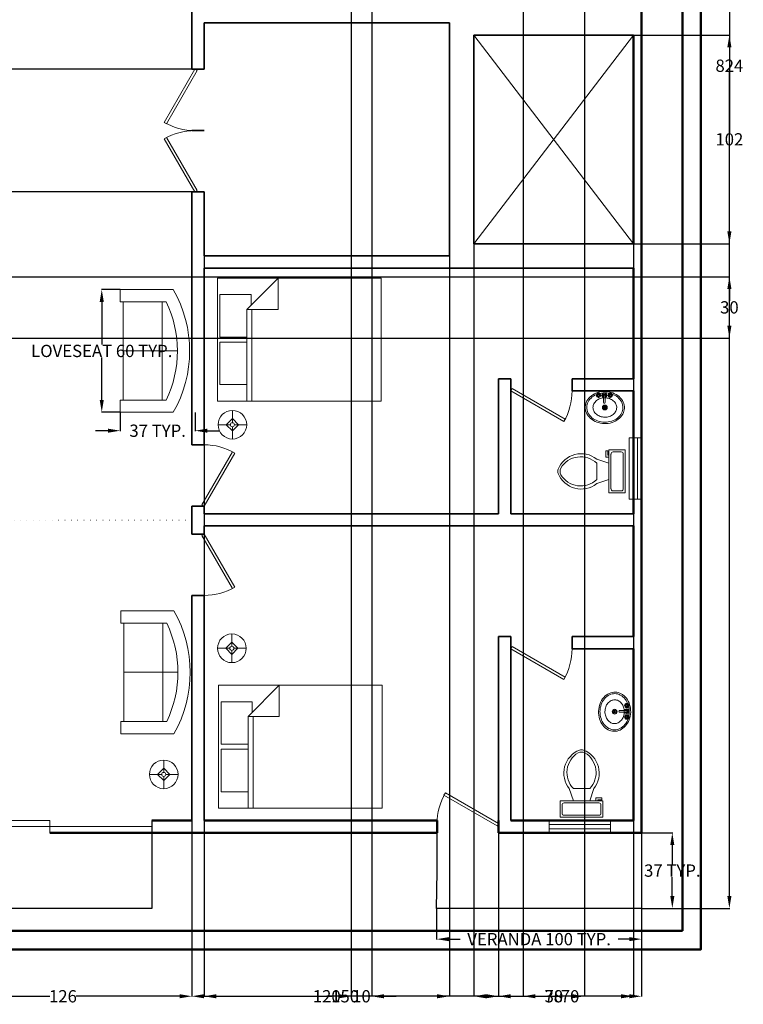
# Model space of a CAD drawing. Units: inches. Extents: x 910 to 1553, y 598 to 1516.
# Tile 2 of 6: x 1198 to 1551, y 598 to 1079. Entities that reach past the tile are written whole.
import ezdxf

# ---------------------------------------------------------------- set-up
doc = ezdxf.new("R2010")
doc.units = ezdxf.units.IN
doc.header["$MEASUREMENT"] = 0
doc.linetypes.add('ACAD_ISO07W100', pattern=[3, 0, -3])
for name, color, linetype, lineweight in [('A-ANNO-DIMS', 2, 'Continuous', 18), ('A-FLOR-BALC', 8, 'Continuous', 25), ('A-FLOR-OPEN', 8, 'Continuous', 13), ('A-FLOR-OVHD', 8, 'ACAD_ISO07W100', 13), ('doors', 2, 'Continuous', 18), ('furniture', 11, 'Continuous', 18), ('Inner wall', 230, 'Continuous', 35), ('outer wall', 231, 'Continuous', 50), ('sanitory', 141, 'Continuous', 18), ('windows', 6, 'Continuous', 18)]:
    doc.layers.add(name, color=color, linetype=linetype, lineweight=lineweight)
doc.styles.get("Standard").update_dxf_attribs({"font": 'arial.ttf'})
doc.dimstyles.get("Standard").update_dxf_attribs({"dimtxt": 6, "dimasz": 6, "dimexe": 0.18, "dimexo": 0.0625, "dimgap": 0.09, "dimtad": 0, "dimtih": 1, "dimtoh": 1, "dimdec": 0, "dimzin": 0, "dimdsep": 46, "dimlunit": 3, "dimtxsty": 'Standard', "dimcen": 0.09, "dimadec": 0, "dimazin": 0, "dimtfac": 1, "dimtdec": 0, "dimtofl": 0, "dimtmove": 0, "dimatfit": 3, "dimfxl": 1, "dimtolj": 1, "dimtzin": 0, "dimarcsym": 0})

# ---------------------------------------------------------------- blocks, each defined once
blk = doc.blocks.new('*U5')
for p, q in [((0, 0), (0, -6)), ((-40, 0), (-40, -6))]:
    blk.add_line(p, q)
blk.add_lwpolyline([(0, 0), (-34.64, 20), (-35.52, 18.48), (-0.88, -1.52)], close=True)
blk.add_arc((0, 0), 40, 150, 180)
blk = doc.blocks.new('*U4')
for p, q in [((0, 0), (0, 6)), ((40, 0), (40, 6))]:
    blk.add_line(p, q)
blk.add_lwpolyline([(0, 0), (34.64, -20), (35.52, -18.48), (0.87, 1.52)], close=True)
blk.add_arc((0, 0), 40, 330, 0)
blk = doc.blocks.new('*U8')
for p, q in [((0, 0), (0, 6)), ((40, 0), (40, 6))]:
    blk.add_line(p, q)
blk.add_lwpolyline([(0, 0), (34.64, -20), (35.52, -18.48), (0.88, 1.52)], close=True)
blk.add_arc((0, 0), 40, 330, 360)
blk = doc.blocks.new('*U6')
for p, q in [((-40, 0), (-40, 6)), ((0, 0), (0, 6))]:
    blk.add_line(p, q)
blk.add_lwpolyline([(0, 0), (-34.64, -20), (-35.52, -18.48), (-0.88, 1.52)], close=True)
blk.add_arc((0, 0), 40, 180, 210)
blk = doc.blocks.new('*U2')
for p, q in [((0, 0), (0, -6)), ((40, 0), (40, -6))]:
    blk.add_line(p, q)
blk.add_lwpolyline([(0, 0), (34.64, 20), (35.52, 18.48), (0.87, -1.52)], close=True)
blk.add_arc((0, 0), 40, 0, 30)
blk = doc.blocks.new('Bed - Queen')
for p, q in [((0, -80.00003), (0, 0)), ((0, 0), (59.99999, 0)), ((59.99999, 0), (59.99999, -80.00003)), ((7.99999, -1.2), (28.79998, -1.2)), ((7.99999, -14.4), (7.99999, -1.2)), ((28.79998, -1.2), (28.79998, -14.4)), ((31.19999, -1.2), (51.99999, -1.2)), ((31.19999, -14.4), (31.19999, -1.2)), ((51.99999, -1.2), (51.99999, -16.4)), ((0, -14.4), (44.8, -14.4)), ((59.99999, -29.6), (44.8, -14.4)), ((44.8, -14.4), (44.8, -29.6)), ((44.8, -16.8), (0, -16.8)), ((51.99999, -16.4), (46.79936, -16.4)), ((44.8, -29.6), (59.99999, -29.6)), ((59.99999, -80.00003), (0, -80.00003))]:
    blk.add_line(p, q)
blk = doc.blocks.new('Lamp - Table')
for p, q in [((0, 7), (0, 1)), ((-1, 0), (-7, 0)), ((0, 3), (-3, 0)), ((-3, 0), (0, -3)), ((3, 0), (0, 3)), ((0, -3), (3, 0)), ((1, 0), (7, 0)), ((0, -1), (0, -7))]:
    blk.add_line(p, q)
for radius in [7, 1]:
    blk.add_circle((0, 0), radius)
blk = doc.blocks.new('Toilet - top')
for p, q in [((9.5, -6), (9.5, -2)), ((-10, -8.5), (-8, -8.5)), ((-10, -9.5), (-10, -8.5)), ((-7, -9.5), (-10, -9.5)), ((-8, -8.5), (-8, -8)), ((-7, -8), (-7, -9.5)), ((-4, -8), (-6, -14)), ((4, -8), (6, -14)), ((4, -14), (-4, -14))]:
    blk.add_line(p, q)
blk.add_lwpolyline([(10.5, -8), (10.5, 0), (-10.5, 0), (-10.5, -8)], close=True)
for points in [[(-9.5, -2), (-9.5, -6)], [(8.5, -1), (-8.5, -1)], [(-8.5, -7), (8.5, -7)]]:
    blk.add_lwpolyline(points)
for centre, radius, start, end in [((-8.62, -1.88), 0.884, 81.8699, 188.1301), ((8.62, -1.88), 0.884, 351.8699, 98.1301), ((-8.62, -6.12), 0.884, 171.8699, 278.1301), ((8.62, -6.12), 0.884, 261.8699, 8.1301), ((3.52, -21.58), 12.17, 141.4691, 247.9714), ((4.2, -21.82), 11.33, 136.3677, 238.9468), ((-3.52, -21.58), 12.17, 292.0284, 38.5307), ((-4.2, -21.82), 11.33, 301.053, 43.6321), ((0, -27.88), 4, 245.7318, 294.2682), ((0, -29), 4, 254.8605, 285.1395)]:
    blk.add_arc(centre, radius, start, end)
blk = doc.blocks.new('Sofa - Roundback Loveseat 5 ft.')
for p, q in [((0, -32.44198), (0, -5.99998)), ((-24, -33.99998), (-24, -11.46958)), ((-23.9998, -13.38178), (23.99986, -13.38178)), ((24.00004, -33.99998), (24.00004, -11.46958)), ((-24, -32.44198), (24.00004, -32.44198))]:
    blk.add_line(p, q)
for points in [[(-24, -33.99998), (-30, -33.99998), (-30, -7.99998)], [(30.00004, -7.99998), (30.00004, -33.99998), (24.00004, -33.99998)]]:
    blk.add_lwpolyline(points)
for centre, radius, start, end in [((0, -60.24998), 60.24998, 60.13715, 119.8628), ((0, -61.38438), 55.38444, 64.32083, 115.6792)]:
    blk.add_arc(centre, radius, start, end)
blk = doc.blocks.new('Faucet - Bathroom top')
for p, q in [((-4.107, 0.125), (-4.375, 0.125)), ((-3.75, 0.4788), (-3.75, 0.75)), ((-3.5, 0.482), (-3.5, 0.75)), ((-3.1461, 0.125), (-2.875, 0.125)), ((3.143, 0.125), (2.875, 0.125)), ((3.5, 0.4788), (3.5, 0.75)), ((3.75, 0.482), (3.75, 0.75)), ((4.1039, 0.125), (4.375, 0.125)), ((-4.1039, -0.125), (-4.375, -0.125)), ((-3.75, -0.4821), (-3.75, -0.75)), ((-3.5, -0.4789), (-3.5, -0.75)), ((-3.143, -0.125), (-2.875, -0.125)), ((-0.5, -0.8639), (-0.5, -4.5)), ((0.5, -4.5), (0.5, -0.8631)), ((3.1461, -0.125), (2.875, -0.125)), ((3.5, -0.4821), (3.5, -0.75)), ((3.75, -0.4789), (3.75, -0.75)), ((4.107, -0.125), (4.375, -0.125))]:
    blk.add_line(p, q)
for centre, radius in [((-3.625, 0), 1.375), ((-4.625, 0), 0.2795), ((-3.625, 0), 0.5), ((-3.625, 1), 0.2795), ((-2.625, 0), 0.2795), ((0, 0), 0.5), ((3.625, 0), 1.375), ((2.625, 0), 0.2795), ((3.625, 0), 0.5), ((3.625, 1), 0.2795), ((4.625, 0), 0.2795), ((-3.625, -1), 0.2795), ((3.625, -1), 0.2795)]:
    blk.add_circle(centre, radius)
for centre, radius, start, end in [((-3.625, 0), 1, 105.2407, 164.2093), ((-3.625, 0), 1, 16.44125, 74.07887), ((0, 0), 1.5, 289.6514, 250.3603), ((0, 0), 1, 300.3431, 239.7554), ((3.625, 0), 1, 106.12, 164.0884), ((3.625, 0), 1, 16.23422, 73.90469), ((-3.625, 0), 1, 196.2342, 253.9047), ((-3.625, 0), 1, 286.12, 344.0884), ((0, -4.5), 0.5, 180, 0), ((3.625, 0), 1, 196.4413, 254.0789), ((3.625, 0), 1, 285.2407, 344.2093)]:
    blk.add_arc(centre, radius, start, end)
blk = doc.blocks.new('Sink - Oval top')
for p, q in [((-1, 0), (1, 0)), ((0, 1), (0, -1))]:
    blk.add_line(p, q)
for points in [[(-12.23, 0.39, 0.117634), (-11.46, -3.36, 0.104469), (-8.88, -6.8, 0.090016), (-5.08, -9.07, 0.08192), (-0.32, -10.02, 0.08192), (4.49, -9.38, 0.090016), (8.42, -7.36, 0.104469), (11.22, -4.09, 0.117634), (12.23, -0.39, 0.117634), (11.46, 3.36, 0.104469), (8.88, 6.8, 0.090016), (5.08, 9.07, 0.08192), (0.32, 10.02, 0.08192), (-4.49, 9.38, 0.090016), (-8.42, 7.36, 0.104469), (-11.22, 4.09, 0.117634)], [(-11.29, 0.16, 0.118622), (-10.52, -3.25, 0.104678), (-8.07, -6.36, 0.089562), (-4.54, -8.37, 0.081185), (-0.13, -9.15, 0.081185), (4.3, -8.49, 0.089562), (7.89, -6.58, 0.104678), (10.42, -3.55, 0.118622), (11.29, -0.16, 0.118622), (10.52, 3.25, 0.104678), (8.07, 6.36, 0.089562), (4.54, 8.37, 0.081185), (0.13, 9.15, 0.081185), (-4.3, 8.49, 0.089562), (-7.89, 6.58, 0.104678), (-10.42, 3.55, 0.118622)], [(-7.42, 0.08, 0.118283), (-6.91, -2.17, 0.104607), (-5.29, -4.21, 0.089718), (-2.97, -5.53, 0.081436), (-0.07, -6.04, 0.081436), (2.84, -5.59, 0.089718), (5.2, -4.33, 0.104607), (6.86, -2.32, 0.118283), (7.42, -0.08, 0.118283), (6.91, 2.17, 0.104607), (5.29, 4.21, 0.089718), (2.97, 5.53, 0.081436), (0.07, 6.04, 0.081436), (-2.84, 5.59, 0.089718), (-5.2, 4.33, 0.104607), (-6.86, 2.32, 0.118283)]]:
    blk.add_lwpolyline(points, format="xyb", close=True)
for radius in [1.5, 1]:
    blk.add_circle((0, 0), radius)
blk = doc.blocks.new('WIN-30X6')
for p, q in [((0, 6), (30, 6)), ((0, 0), (0, 6)), ((30, 6), (30, 0)), ((0, 4), (30, 4)), ((30, 2), (0, 2)), ((30, 0), (0, 0))]:
    blk.add_line(p, q)
blk = doc.blocks.new('VERANDA-EDGE-DEEP')
for p, q in [((0.23, 17.99), (0.23, 36.98)), ((100.23, 36.98), (100.23, 17.99)), ((0, 0), (0.23, 17.99)), ((100.23, 17.99), (100.23, 0)), ((100.23, 0), (0, 0))]:
    blk.add_line(p, q)
blk = doc.blocks.new('*D41')
at = {"layer": 'A-ANNO-DIMS', "color": 0, "lineweight": -2, "transparency": 16777216}
for p, q in [((1246.6, 947.53), (1237.49, 947.53)), ((1237.67, 941.53), (1237.67, 920.72)), ((1237.67, 893.53), (1237.67, 914.33)), ((1246.6, 887.53), (1237.49, 887.53))]:
    blk.add_line(p, q, dxfattribs=at)
for points in [[(1236.67, 941.53), (1238.67, 941.53), (1237.67, 947.53)], [(1236.67, 893.53), (1238.67, 893.53), (1237.67, 887.53)]]:
    blk.add_solid(points, dxfattribs=at)
at = {"layer": 'Defpoints', "color": 0, "lineweight": -2, "transparency": 16777216}
for p in [(1246.67, 947.53), (1237.67, 887.53), (1246.67, 887.53)]:
    blk.add_point(p, dxfattribs=at)
at = {"layer": 'A-ANNO-DIMS', "color": 0, "transparency": 16777216, "insert": (1237.67, 917.53), "char_height": 6, "attachment_point": 5}
blk.add_mtext('\\A1;LOVESEAT 60 TYP.', dxfattribs=at)
blk = doc.blocks.new('*D42')
at = {"layer": 'A-ANNO-DIMS', "color": 0, "lineweight": -2, "transparency": 16777216}
for p, q in [((1246.67, 887.46), (1246.67, 878.35)), ((1283.33, 887.46), (1283.33, 878.35)), ((1240.67, 878.53), (1234.67, 878.53)), ((1289.33, 878.53), (1295.33, 878.53))]:
    blk.add_line(p, q, dxfattribs=at)
for points in [[(1240.67, 879.53), (1240.67, 877.53), (1246.67, 878.53)], [(1289.33, 879.53), (1289.33, 877.53), (1283.33, 878.53)]]:
    blk.add_solid(points, dxfattribs=at)
at = {"layer": 'Defpoints', "color": 0, "lineweight": -2, "transparency": 16777216}
for p in [(1246.67, 887.53), (1283.33, 887.53), (1283.33, 878.53)]:
    blk.add_point(p, dxfattribs=at)
at = {"layer": 'A-ANNO-DIMS', "color": 0, "transparency": 16777216, "insert": (1265, 878.53), "char_height": 6, "attachment_point": 5}
blk.add_mtext('\\A1;37 TYP.', dxfattribs=at)
blk = doc.blocks.new('*D47')
at = {"layer": 'A-ANNO-DIMS', "color": 0, "lineweight": -2, "transparency": 16777216}
for p, q in [((1401.47, 644.93), (1401.47, 629.78)), ((1501.7, 644.93), (1501.7, 629.78)), ((1407.47, 629.96), (1412.98, 629.96)), ((1495.7, 629.96), (1490.19, 629.96))]:
    blk.add_line(p, q, dxfattribs=at)
for points in [[(1407.47, 630.96), (1407.47, 628.96), (1401.47, 629.96)], [(1495.7, 630.96), (1495.7, 628.96), (1501.7, 629.96)]]:
    blk.add_solid(points, dxfattribs=at)
at = {"layer": 'Defpoints', "color": 0, "lineweight": -2, "transparency": 16777216}
for p in [(1401.47, 644.99), (1501.7, 644.99), (1501.7, 629.96)]:
    blk.add_point(p, dxfattribs=at)
at = {"layer": 'A-ANNO-DIMS', "color": 0, "transparency": 16777216, "insert": (1451.59, 629.96), "char_height": 6, "attachment_point": 5}
blk.add_mtext('\\A1;VERANDA 100 TYP.', dxfattribs=at)
blk = doc.blocks.new('*D48')
at = {"layer": 'A-ANNO-DIMS', "color": 0, "lineweight": -2, "transparency": 16777216}
for p, q in [((1501.76, 681.97), (1516.92, 681.97)), ((1516.74, 675.97), (1516.74, 666.64)), ((1516.74, 650.99), (1516.74, 660.33)), ((1501.76, 644.99), (1516.92, 644.99))]:
    blk.add_line(p, q, dxfattribs=at)
for points in [[(1515.74, 675.97), (1517.74, 675.97), (1516.74, 681.97)], [(1515.74, 650.99), (1517.74, 650.99), (1516.74, 644.99)]]:
    blk.add_solid(points, dxfattribs=at)
at = {"layer": 'Defpoints', "color": 0, "lineweight": -2, "transparency": 16777216}
for p in [(1501.7, 681.97), (1516.74, 681.97), (1501.7, 644.99)]:
    blk.add_point(p, dxfattribs=at)
at = {"layer": 'A-ANNO-DIMS', "color": 0, "transparency": 16777216, "insert": (1516.74, 663.48), "char_height": 6, "attachment_point": 5}
blk.add_mtext('\\A1;37 TYP.', dxfattribs=at)
blk = doc.blocks.new('*D56')
at = {"layer": 'A-ANNO-DIMS', "color": 0, "lineweight": -2, "transparency": 16777216}
for p, q in [((1501.76, 1468.95), (1544.83, 1468.95)), ((1544.65, 1462.95), (1544.65, 1060.13)), ((1544.65, 650.99), (1544.65, 1053.82)), ((1501.76, 644.99), (1544.83, 644.99))]:
    blk.add_line(p, q, dxfattribs=at)
for points in [[(1543.65, 1462.95), (1545.65, 1462.95), (1544.65, 1468.95)], [(1543.65, 650.99), (1545.65, 650.99), (1544.65, 644.99)]]:
    blk.add_solid(points, dxfattribs=at)
at = {"layer": 'Defpoints', "color": 0, "lineweight": -2, "transparency": 16777216}
for p in [(1501.7, 1468.95), (1544.65, 1468.95), (1501.7, 644.99)]:
    blk.add_point(p, dxfattribs=at)
at = {"layer": 'A-ANNO-DIMS', "color": 0, "transparency": 16777216, "insert": (1544.65, 1056.97), "char_height": 6, "attachment_point": 5}
blk.add_mtext('\\A1;824', dxfattribs=at)
blk = doc.blocks.new('*D59')
at = {"layer": 'A-ANNO-DIMS', "color": 0, "lineweight": -2, "transparency": 16777216}
for p, q in [((1155.7, 687.91), (1155.7, 601.86)), ((1281.7, 687.91), (1281.7, 601.86)), ((1161.7, 602.04), (1212.27, 602.04)), ((1275.7, 602.04), (1225.13, 602.04))]:
    blk.add_line(p, q, dxfattribs=at)
for points in [[(1161.7, 603.04), (1161.7, 601.04), (1155.7, 602.04)], [(1275.7, 603.04), (1275.7, 601.04), (1281.7, 602.04)]]:
    blk.add_solid(points, dxfattribs=at)
at = {"layer": 'Defpoints', "color": 0, "lineweight": -2, "transparency": 16777216}
for p in [(1155.7, 687.97), (1281.7, 687.97), (1281.7, 602.04)]:
    blk.add_point(p, dxfattribs=at)
at = {"layer": 'A-ANNO-DIMS', "color": 0, "transparency": 16777216, "insert": (1218.7, 602.04), "char_height": 6, "attachment_point": 5}
blk.add_mtext('\\A1;126', dxfattribs=at)
blk = doc.blocks.new('*D60')
at = {"layer": 'A-ANNO-DIMS', "color": 0, "lineweight": -2, "transparency": 16777216}
for p, q in [((1281.7, 687.91), (1281.7, 601.86)), ((1431.7, 681.91), (1431.7, 601.86)), ((1287.7, 602.04), (1350.27, 602.04)), ((1425.7, 602.04), (1363.13, 602.04))]:
    blk.add_line(p, q, dxfattribs=at)
for points in [[(1287.7, 603.04), (1287.7, 601.04), (1281.7, 602.04)], [(1425.7, 603.04), (1425.7, 601.04), (1431.7, 602.04)]]:
    blk.add_solid(points, dxfattribs=at)
at = {"layer": 'Defpoints', "color": 0, "lineweight": -2, "transparency": 16777216}
for p in [(1281.7, 687.97), (1431.7, 681.97), (1431.7, 602.04)]:
    blk.add_point(p, dxfattribs=at)
at = {"layer": 'A-ANNO-DIMS', "color": 0, "transparency": 16777216, "insert": (1356.7, 602.04), "char_height": 6, "attachment_point": 5}
blk.add_mtext('\\A1;150', dxfattribs=at)
blk = doc.blocks.new('*D61')
at = {"layer": 'A-ANNO-DIMS', "color": 0, "lineweight": -2, "transparency": 16777216}
for p, q in [((1431.7, 681.91), (1431.7, 601.86)), ((1501.7, 681.91), (1501.7, 601.86)), ((1437.7, 602.04), (1462.35, 602.04)), ((1495.7, 602.04), (1471.05, 602.04))]:
    blk.add_line(p, q, dxfattribs=at)
for points in [[(1437.7, 603.04), (1437.7, 601.04), (1431.7, 602.04)], [(1495.7, 603.04), (1495.7, 601.04), (1501.7, 602.04)]]:
    blk.add_solid(points, dxfattribs=at)
at = {"layer": 'Defpoints', "color": 0, "lineweight": -2, "transparency": 16777216}
for p in [(1431.7, 681.97), (1501.7, 681.97), (1501.7, 602.04)]:
    blk.add_point(p, dxfattribs=at)
at = {"layer": 'A-ANNO-DIMS', "color": 0, "transparency": 16777216, "insert": (1466.7, 602.04), "char_height": 6, "attachment_point": 5}
blk.add_mtext('\\A1;70', dxfattribs=at)
blk = doc.blocks.new('*D73')
at = {"layer": 'A-ANNO-DIMS', "color": 0, "lineweight": -2, "transparency": 16777216}
for p, q in [((1443.82, 1359.91), (1443.82, 601.86)), ((1473.82, 1359.91), (1473.82, 601.86)), ((1449.82, 602.04), (1454.45, 602.04)), ((1467.82, 602.04), (1463.2, 602.04))]:
    blk.add_line(p, q, dxfattribs=at)
for points in [[(1449.82, 603.04), (1449.82, 601.04), (1443.82, 602.04)], [(1467.82, 603.04), (1467.82, 601.04), (1473.82, 602.04)]]:
    blk.add_solid(points, dxfattribs=at)
at = {"layer": 'Defpoints', "color": 0, "lineweight": -2, "transparency": 16777216}
for p in [(1443.82, 1359.97), (1473.82, 1359.97), (1473.82, 602.04)]:
    blk.add_point(p, dxfattribs=at)
at = {"layer": 'A-ANNO-DIMS', "color": 0, "transparency": 16777216, "insert": (1458.82, 602.04), "char_height": 6, "attachment_point": 5}
blk.add_mtext('\\A1;30', dxfattribs=at)
blk = doc.blocks.new('*D76')
at = {"layer": 'A-ANNO-DIMS', "color": 0, "lineweight": -2, "transparency": 16777216}
for p, q in [((1089.76, 953.83), (1544.83, 953.83)), ((1544.65, 947.83), (1544.65, 941.98)), ((1544.65, 929.83), (1544.65, 935.67)), ((1089.76, 923.83), (1544.83, 923.83))]:
    blk.add_line(p, q, dxfattribs=at)
for points in [[(1543.65, 947.83), (1545.65, 947.83), (1544.65, 953.83)], [(1543.65, 929.83), (1545.65, 929.83), (1544.65, 923.83)]]:
    blk.add_solid(points, dxfattribs=at)
at = {"layer": 'Defpoints', "color": 0, "lineweight": -2, "transparency": 16777216}
for p in [(1089.7, 953.83), (1544.65, 953.83), (1089.7, 923.83)]:
    blk.add_point(p, dxfattribs=at)
at = {"layer": 'A-ANNO-DIMS', "color": 0, "transparency": 16777216, "insert": (1544.65, 938.83), "char_height": 6, "attachment_point": 5}
blk.add_mtext('\\A1;30', dxfattribs=at)
blk = doc.blocks.new('*D81')
at = {"layer": 'A-ANNO-DIMS', "color": 0, "lineweight": -2, "transparency": 16777216}
for p, q in [((1359.700482, 1083.906924), (1359.700482, 601.863289)), ((1369.700482, 1083.906924), (1369.700482, 601.863289)), ((1353.700482, 602.043289), (1347.700482, 602.043289)), ((1375.700482, 602.043289), (1381.700482, 602.043289))]:
    blk.add_line(p, q, dxfattribs=at)
for points in [[(1353.700482, 603.043289), (1353.700482, 601.043289), (1359.700482, 602.043289)], [(1375.700482, 603.043289), (1375.700482, 601.043289), (1369.700482, 602.043289)]]:
    blk.add_solid(points, dxfattribs=at)
at = {"layer": 'Defpoints', "color": 0, "lineweight": -2, "transparency": 16777216}
for p in [(1359.700482, 1083.969424), (1369.700482, 1083.969424), (1369.700482, 602.043289)]:
    blk.add_point(p, dxfattribs=at)
at = {"layer": 'A-ANNO-DIMS', "color": 0, "transparency": 16777216, "insert": (1364.700482, 602.043289), "char_height": 6, "attachment_point": 5}
blk.add_mtext('\\A1;10', dxfattribs=at)
blk = doc.blocks.new('*D82')
at = {"layer": 'A-ANNO-DIMS', "color": 0, "lineweight": -2, "transparency": 16777216}
for p, q in [((1287.7, 963.91), (1287.7, 601.86)), ((1407.7, 963.91), (1407.7, 601.86)), ((1293.7, 602.04), (1341.27, 602.04)), ((1401.7, 602.04), (1354.13, 602.04))]:
    blk.add_line(p, q, dxfattribs=at)
for points in [[(1293.7, 603.04), (1293.7, 601.04), (1287.7, 602.04)], [(1401.7, 603.04), (1401.7, 601.04), (1407.7, 602.04)]]:
    blk.add_solid(points, dxfattribs=at)
at = {"layer": 'Defpoints', "color": 0, "lineweight": -2, "transparency": 16777216}
for p in [(1287.7, 963.97), (1407.7, 963.97), (1407.7, 602.04)]:
    blk.add_point(p, dxfattribs=at)
at = {"layer": 'A-ANNO-DIMS', "color": 0, "transparency": 16777216, "insert": (1347.7, 602.04), "char_height": 6, "attachment_point": 5}
blk.add_mtext('\\A1;120', dxfattribs=at)
blk = doc.blocks.new('*D83')
at = {"layer": 'A-ANNO-DIMS', "color": 0, "lineweight": -2, "transparency": 16777216}
for p, q in [((1419.7, 969.91), (1419.7, 601.86)), ((1497.7, 969.91), (1497.7, 601.86)), ((1425.7, 602.04), (1454.33, 602.04)), ((1491.7, 602.04), (1463.07, 602.04))]:
    blk.add_line(p, q, dxfattribs=at)
for points in [[(1425.7, 603.04), (1425.7, 601.04), (1419.7, 602.04)], [(1491.7, 603.04), (1491.7, 601.04), (1497.7, 602.04)]]:
    blk.add_solid(points, dxfattribs=at)
at = {"layer": 'Defpoints', "color": 0, "lineweight": -2, "transparency": 16777216}
for p in [(1419.7, 969.97), (1497.7, 969.97), (1497.7, 602.04)]:
    blk.add_point(p, dxfattribs=at)
at = {"layer": 'A-ANNO-DIMS', "color": 0, "transparency": 16777216, "insert": (1458.7, 602.04), "char_height": 6, "attachment_point": 5}
blk.add_mtext('\\A1;78', dxfattribs=at)
blk = doc.blocks.new('*D84')
at = {"layer": 'A-ANNO-DIMS', "color": 0, "lineweight": -2, "transparency": 16777216}
for p, q in [((1497.76, 1071.97), (1544.83, 1071.97)), ((1544.65, 1065.97), (1544.65, 1024.12)), ((1544.65, 975.97), (1544.65, 1017.82)), ((1497.76, 969.97), (1544.83, 969.97))]:
    blk.add_line(p, q, dxfattribs=at)
for points in [[(1543.65, 1065.97), (1545.65, 1065.97), (1544.65, 1071.97)], [(1543.65, 975.97), (1545.65, 975.97), (1544.65, 969.97)]]:
    blk.add_solid(points, dxfattribs=at)
at = {"layer": 'Defpoints', "color": 0, "lineweight": -2, "transparency": 16777216}
for p in [(1497.7, 1071.97), (1544.65, 1071.97), (1497.7, 969.97)]:
    blk.add_point(p, dxfattribs=at)
at = {"layer": 'A-ANNO-DIMS', "color": 0, "transparency": 16777216, "insert": (1544.65, 1020.97), "char_height": 6, "attachment_point": 5}
blk.add_mtext('\\A1;102', dxfattribs=at)
blk = doc.blocks.new('*D85')
at = {"layer": 'A-ANNO-DIMS', "color": 0, "lineweight": -2, "transparency": 16777216}
for p, q in [((1287.64, 1055.24), (916.34, 1055.24)), ((916.52, 1049.24), (916.52, 1028.4)), ((916.52, 1001.24), (916.52, 1022.09)), ((1287.64, 995.24), (916.34, 995.24))]:
    blk.add_line(p, q, dxfattribs=at)
for points in [[(915.52, 1049.24), (917.52, 1049.24), (916.52, 1055.24)], [(915.52, 1001.24), (917.52, 1001.24), (916.52, 995.24)]]:
    blk.add_solid(points, dxfattribs=at)
at = {"layer": 'Defpoints', "color": 0, "lineweight": -2, "transparency": 16777216}
for p in [(916.52, 1055.24), (1287.7, 1055.24), (1287.7, 995.24)]:
    blk.add_point(p, dxfattribs=at)
at = {"layer": 'A-ANNO-DIMS', "color": 0, "transparency": 16777216, "insert": (916.52, 1025.24), "char_height": 6, "attachment_point": 5}
blk.add_mtext('\\A1;60', dxfattribs=at)

msp = doc.modelspace()

# ---------------------------------------------------------------- linework, layer by layer
at = {"layer": 'A-FLOR-BALC'}
for p, q in [((1262.234, 687.969), (1262.234, 662.984)), ((1262.234, 662.984), (1262.234, 644.993)), ((1262.234, 644.993), (1162.004, 644.993))]:
    msp.add_line(p, q, dxfattribs=at)
at = {"layer": 'A-FLOR-OPEN'}
for p, q in [((1419.7, 1071.969), (1497.7, 969.969)), ((1497.7, 1071.969), (1419.7, 969.969))]:
    msp.add_line(p, q, dxfattribs=at)
at = {"layer": 'A-FLOR-OVHD'}
msp.add_line((1281.7, 834.815), (1155.7, 834.815), dxfattribs=at)
at = {"layer": 'doors'}
for p, q in [((1155.7, 687.969), (1212.234, 687.969)), ((1162.234, 684.969), (1262.234, 684.969)), ((1212.234, 684.969), (1212.234, 687.969)), ((1212.234, 687.969), (1212.234, 681.969)), ((1262.234, 681.969), (1262.234, 684.969)), ((1212.234, 681.969), (1262.234, 681.969))]:
    msp.add_line(p, q, dxfattribs=at)
at = {"layer": 'Inner wall'}
for p, q in [((1281.7, 1111.545), (1281.7, 1055.242)), ((1407.7, 1077.969), (1287.7, 1077.969)), ((1287.7, 1077.969), (1287.7, 1055.242)), ((1407.7, 963.969), (1407.7, 1077.969)), ((1419.7, 969.969), (1419.7, 1071.969)), ((1431.7, 1071.969), (1419.7, 1071.969)), ((1431.7, 1071.969), (1437.7, 1071.969)), ((1497.7, 1071.969), (1437.7, 1071.969)), ((1281.7, 995.242), (1281.7, 963.969)), ((1281.7, 995.242), (1281.7, 871.637)), ((1287.7, 995.242), (1287.7, 963.969)), ((1419.7, 969.969), (1431.7, 969.969)), ((1431.7, 969.969), (1437.7, 969.969)), ((1437.7, 969.969), (1497.7, 969.969)), ((1287.7, 963.969), (1407.7, 963.969)), ((1287.7, 957.969), (1497.7, 957.969)), ((1287.7, 957.969), (1287.7, 871.637)), ((1431.7, 837.969), (1431.7, 903.969)), ((1431.7, 903.969), (1437.7, 903.969)), ((1437.7, 837.969), (1437.7, 903.969)), ((1467.7, 903.969), (1497.7, 903.969)), ((1467.7, 897.969), (1497.7, 897.969)), ((1281.7, 841.637), (1281.7, 827.992)), ((1287.7, 841.637), (1287.7, 837.969)), ((1287.7, 837.969), (1431.7, 837.969)), ((1437.7, 837.969), (1497.7, 837.969)), ((1281.7, 831.969), (1281.7, 827.992)), ((1287.7, 831.969), (1287.7, 827.992)), ((1287.7, 831.969), (1497.7, 831.969)), ((1281.7, 797.992), (1281.7, 687.969)), ((1287.7, 797.992), (1287.7, 687.969)), ((1431.7, 687.969), (1431.7, 777.969)), ((1431.7, 777.969), (1437.7, 777.969)), ((1437.7, 687.969), (1437.7, 777.969)), ((1467.7, 777.969), (1497.7, 777.969)), ((1467.7, 771.969), (1497.7, 771.969))]:
    msp.add_line(p, q, dxfattribs=at)
for points in [[(1281.7, 1055.242), (1287.7, 1055.242)], [(1287.7, 1025.242), (1281.7, 1025.242)], [(1281.7, 1025.242), (1287.7, 1025.242)], [(1287.7, 995.242), (1281.7, 995.242)], [(1437.7, 897.969), (1437.7, 903.969)], [(1467.7, 903.969), (1467.7, 897.969)], [(1281.7, 871.637), (1287.7, 871.637)], [(1287.7, 841.637), (1281.7, 841.637)], [(1281.7, 827.992), (1287.7, 827.992)], [(1287.7, 797.992), (1281.7, 797.992)], [(1437.7, 771.969), (1437.7, 777.969)], [(1467.7, 777.969), (1467.7, 771.969)]]:
    msp.add_lwpolyline(points, dxfattribs=at)
at = {"layer": 'outer wall'}
for p, q in [((1521.7, 633.969), (1521.7, 1479.969)), ((1501.7, 681.969), (1501.7, 1449.969)), ((1497.7, 969.969), (1497.7, 1071.969)), ((1497.7, 903.969), (1497.7, 957.969)), ((1497.7, 837.969), (1497.7, 897.969)), ((1497.7, 777.969), (1497.7, 831.969)), ((1497.7, 687.969), (1497.7, 771.969)), ((1262.234, 687.969), (1281.7, 687.969)), ((1287.7, 687.969), (1401.7, 687.969)), ((1437.7, 687.969), (1497.7, 687.969)), ((1212.234, 681.969), (1401.7, 681.969)), ((1431.7, 681.969), (1497.7, 681.969)), ((1497.7, 681.969), (1501.7, 681.969)), ((939.7, 633.969), (1521.7, 633.969))]:
    msp.add_line(p, q, dxfattribs=at)
msp.add_lwpolyline([(1530.7, 1488.969), (930.7, 1488.969), (930.7, 624.969), (1530.7, 624.969)], close=True, dxfattribs=at)
for points in [[(1401.7, 681.969), (1401.7, 687.969)], [(1431.7, 687.969), (1431.7, 681.969)]]:
    msp.add_lwpolyline(points, dxfattribs=at)

# ---------------------------------------------------------------- block references
at = {"layer": 'A-FLOR-BALC'}
msp.add_blockref('VERANDA-EDGE-DEEP', (1401.47, 644.993), dxfattribs=at)
at = {"layer": 'doors', "xscale": 0.75, "yscale": 0.75, "zscale": 0.75, "rotation": 90}
for name, p in [('*U5', (1283.2, 1055.242)), ('*U2', (1283.2, 995.242)), ('*U4', (1287.7, 841.637)), ('*U6', (1287.7, 827.992))]:
    msp.add_blockref(name, p, dxfattribs=at)
at = {"layer": 'doors', "xscale": 0.75, "yscale": 0.75, "zscale": 0.75}
for name, p in [('*U4', (1437.7, 897.969)), ('*U8', (1437.7, 771.969)), ('*U5', (1431.7, 686.469))]:
    msp.add_blockref(name, p, dxfattribs=at)
at = {"layer": 'furniture'}
for name, p, rotation in [('Bed - Queen', (1294.293, 893.043), 90), ('Sofa - Roundback Loveseat 5 ft.', (1280.666, 917.526), 270), ('Sofa - Roundback Loveseat 5 ft.', (1280.936, 760.406), 270), ('Bed - Queen', (1294.854, 694.05), 90)]:
    msp.add_blockref(name, p, dxfattribs=dict(at, rotation=rotation))
for p in [(1301.578, 881.455), (1301.309, 772.148), (1267.992, 710.507)]:
    msp.add_blockref('Lamp - Table', p, dxfattribs=at)
at = {"layer": 'sanitory', "xscale": 0.7833329843755676, "yscale": 0.7833329843755676, "zscale": 0.7833329843755676}
for name, p, rotation in [('Sink - Oval top', (1483.736, 889.873), 180), ('Sink - Oval top', (1488.52, 741.155), 90), ('Faucet - Bathroom top', (1494.488, 741.398), 270)]:
    msp.add_blockref(name, p, dxfattribs=dict(at, rotation=rotation))
msp.add_blockref('Faucet - Bathroom top', (1483.493, 895.84), dxfattribs=at)
at = {"layer": 'sanitory'}
for p, rotation in [((1493.744, 858.642), 270), ((1472.332, 689.551), 180)]:
    msp.add_blockref('Toilet - top', p, dxfattribs=dict(at, rotation=rotation))
at = {"layer": 'windows'}
for p, rotation in [((1501.7, 845.058), 90.00000000000082), ((1486.473, 687.969), 180)]:
    msp.add_blockref('WIN-30X6', p, dxfattribs=dict(at, rotation=rotation))

# ---------------------------------------------------------------- dimensions: what is measured, and where the dimension line sits
at = {"layer": 'A-ANNO-DIMS'}
for base, p1, p2, picture, middle in [((1544.65, 1468.955), (1501.7, 644.993), (1501.7, 1468.955), '*D56', (1544.65, 1056.974)), ((1544.65, 1071.969), (1497.7, 969.969), (1497.7, 1071.969), '*D84', (1544.65, 1020.969)), ((916.52, 1055.242), (1287.7, 995.242), (1287.7, 1055.242), '*D85', (916.52, 1025.242)), ((1544.65, 953.828), (1089.7, 923.828), (1089.7, 953.828), '*D76', (1544.65, 938.828))]:
    dim = msp.add_linear_dim(base=base, p1=p1, p2=p2, angle=90, dimstyle='Standard', override={"dimdec": 0, "dimlfac": 1, "dimrnd": 0, "dimzin": 0, "dimdsep": 46, "dimlunit": 2}, dxfattribs=at)
    dim.commit()
    dim.dimension.update_dxf_attribs({"geometry": picture, "text_midpoint": middle})
for base, p1, p2, picture, middle in [((1473.82, 602.043), (1443.82, 1359.969), (1473.82, 1359.969), '*D73', (1458.82, 602.043)), ((1369.7, 602.043), (1359.7, 1083.969), (1369.7, 1083.969), '*D81', (1364.7, 602.043)), ((1497.7, 602.043), (1419.7, 969.969), (1497.7, 969.969), '*D83', (1458.7, 602.043)), ((1407.7, 602.043), (1287.7, 963.969), (1407.7, 963.969), '*D82', (1347.7, 602.043)), ((1281.7, 602.043), (1155.7, 687.969), (1281.7, 687.969), '*D59', (1218.7, 602.043)), ((1431.7, 602.043), (1281.7, 687.969), (1431.7, 681.969), '*D60', (1356.7, 602.043)), ((1501.7, 602.043), (1431.7, 681.969), (1501.7, 681.969), '*D61', (1466.7, 602.043))]:
    dim = msp.add_linear_dim(base=base, p1=p1, p2=p2, dimstyle='Standard', override={"dimdec": 0, "dimlfac": 1, "dimrnd": 0, "dimzin": 0, "dimdsep": 46, "dimlunit": 2}, dxfattribs=at)
    dim.commit()
    dim.dimension.update_dxf_attribs({"geometry": picture, "text_midpoint": middle})
for base, p1, p2, angle, text, picture, middle in [((1237.666, 887.525), (1246.666, 947.526), (1246.666, 887.525), 270, 'LOVESEAT <> TYP.', '*D41', (1237.666, 917.526)), ((1516.735, 681.969), (1501.7, 644.993), (1501.7, 681.969), 90, '<> TYP.', '*D48', (1516.735, 663.481))]:
    dim = msp.add_linear_dim(base=base, p1=p1, p2=p2, angle=angle, text=text, dimstyle='Standard', override={"dimdec": 0, "dimlfac": 1, "dimrnd": 0, "dimzin": 0, "dimdsep": 46, "dimlunit": 2}, dxfattribs=at)
    dim.commit()
    dim.dimension.update_dxf_attribs({"geometry": picture, "text_midpoint": middle})
for base, p1, p2, text, picture, middle in [((1283.333, 878.525), (1246.666, 887.525), (1283.333, 887.525), '<> TYP.', '*D42', (1264.999, 878.525)), ((1501.7, 629.959), (1401.47, 644.993), (1501.7, 644.993), 'VERANDA <> TYP.', '*D47', (1451.585, 629.959))]:
    dim = msp.add_linear_dim(base=base, p1=p1, p2=p2, text=text, dimstyle='Standard', override={"dimdec": 0, "dimlfac": 1, "dimrnd": 0, "dimzin": 0, "dimdsep": 46, "dimlunit": 2}, dxfattribs=at)
    dim.commit()
    dim.dimension.update_dxf_attribs({"geometry": picture, "text_midpoint": middle})

doc.saveas('drawing.dxf')
